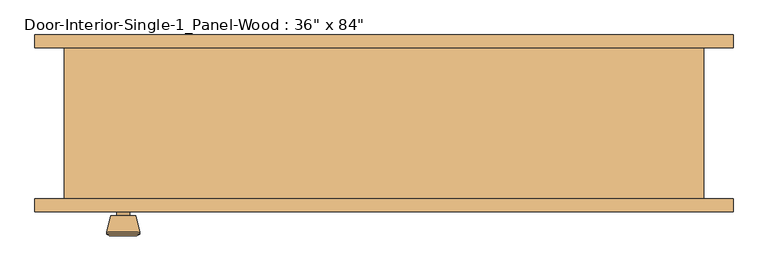
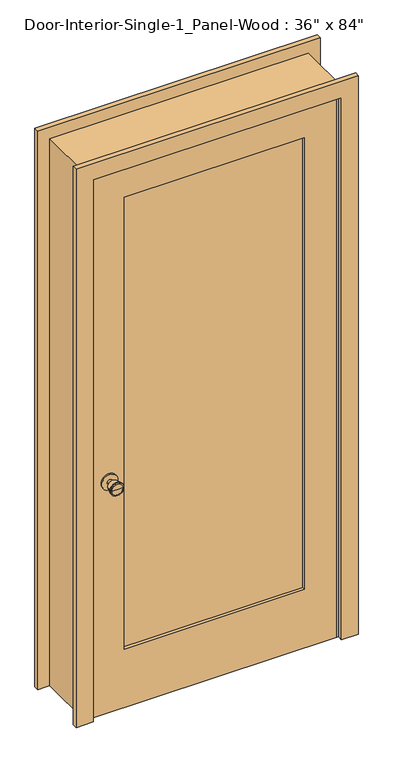
"""IFC4 building model written with IfcOpenShell, lengths in millimetres: door geometry."""

from ifc_helpers import new_model, si_unit, point, frame, frame_2d, origin, place, context, project, spatial, polyline, circle_curve, trimmed, segment, composite_curve, outline, extrude, faceted_brep, source, transform, mapped, element, save
from ifc_brep_helpers import plane_surface, cylinder_surface, revolved_surface, advanced_brep


def door_868ee8a9(model_context):
    return source(origin(), model_context, "Body", "SolidModel", [
        advanced_brep(
        [(-393.7, -70.2, 914.4), (-403.7, -70.2, 914.4), (-383.7, -70.2, 914.4), (-373.2241324, -21.2, 914.4), (-414.1758676, -21.2, 914.4), (-393.7, -21.2, 914.4), (-368.7, -23.0278681, 914.4), (-418.7, -23.0278681, 914.4), (-368.7, -26.4915463, 914.4), (-418.7, -26.4915463, 914.4), (-375.063764, -51.2, 914.4), (-412.336236, -51.2, 914.4), (-383.7, -51.2, 914.4), (-403.7, -51.2, 914.4)],
        [
            (0, 1),
            (1, 2, circle_curve(frame((-393.7, -70.2, 914.4), z_axis=(0.0, -1.0, 0.0), x_axis=(-1.0, 0.0, 0.0)), 10.0)),
            (2, 0),
            (2, 1, circle_curve(frame((-393.7, -70.2, 914.4), z_axis=(0.0, -1.0, 0.0), x_axis=(-1.0, 0.0, 0.0)), 10.0)),
            (3, 4, circle_curve(frame((-393.7, -21.2, 914.4), z_axis=(0.0, 1.0, 0.0), x_axis=(-1.0, 0.0, 0.0)), 20.4758676)),
            (4, 5),
            (5, 3),
            (4, 3, circle_curve(frame((-393.7, -21.2, 914.4), z_axis=(0.0, 1.0, 0.0), x_axis=(-1.0, 0.0, 0.0)), 20.4758676)),
            (6, 7, circle_curve(frame((-393.7, -23.0278681, 914.4), z_axis=(0.0, 1.0, 0.0), x_axis=(-1.0, 0.0, 0.0)), 25.0)),
            (7, 4),
            (3, 6),
            (7, 6, circle_curve(frame((-393.7, -23.0278681, 914.4), z_axis=(0.0, 1.0, 0.0), x_axis=(-1.0, 0.0, 0.0)), 25.0)),
            (8, 9, circle_curve(frame((-393.7, -26.4915463, 914.4), z_axis=(0.0, 1.0, 0.0), x_axis=(-1.0, 0.0, 0.0)), 25.0)),
            (9, 7),
            (6, 8),
            (9, 8, circle_curve(frame((-393.7, -26.4915463, 914.4), z_axis=(0.0, 1.0, 0.0), x_axis=(-1.0, 0.0, 0.0)), 25.0)),
            (10, 11, circle_curve(frame((-393.7, -51.2, 914.4), z_axis=(0.0, 1.0, 0.0), x_axis=(-1.0, 0.0, 0.0)), 18.636236)),
            (11, 9),
            (8, 10),
            (11, 10, circle_curve(frame((-393.7, -51.2, 914.4), z_axis=(0.0, 1.0, 0.0), x_axis=(-1.0, 0.0, 0.0)), 18.636236)),
            (12, 13, circle_curve(frame((-393.7, -51.2, 914.4), z_axis=(0.0, 1.0, 0.0), x_axis=(-1.0, 0.0, 0.0)), 10.0)),
            (13, 11),
            (10, 12),
            (13, 12, circle_curve(frame((-393.7, -51.2, 914.4), z_axis=(0.0, 1.0, 0.0), x_axis=(-1.0, 0.0, 0.0)), 10.0)),
            (1, 13),
            (12, 2),
        ],
        [
            plane_surface(frame((-393.7, -70.2, 914.4), z_axis=(0.0, -1.0, 0.0), x_axis=(-1.0, 0.0, 0.0))),
            plane_surface(frame((-393.7, -21.2, 914.4), z_axis=(0.0, 1.0, 0.0), x_axis=(-1.0, 0.0, 0.0))),
            revolved_surface(polyline([(-414.1758676, -21.2, 914.4), (-418.7, -23.0278681, 914.4)]), (-393.7, -70.2, 914.4), (0.0, -1.0, 0.0)),
            cylinder_surface(frame((-393.7, -70.2, 914.4), z_axis=(0.0, -1.0, 0.0), x_axis=(-1.0, 0.0, 0.0)), 25.0),
            revolved_surface(polyline([(-418.7, -26.4915463, 914.4), (-412.336236, -51.2, 914.4)]), (-393.7, -70.2, 914.4), (0.0, -1.0, 0.0)),
            plane_surface(frame((-393.7, -51.2, 914.4), z_axis=(0.0, -1.0, 0.0), x_axis=(-1.0, 0.0, 0.0))),
            cylinder_surface(frame((-393.7, -70.2, 914.4), z_axis=(0.0, -1.0, 0.0), x_axis=(-1.0, 0.0, 0.0)), 10.0),
        ],
        [
            (0, [[1, 2, 3]]),
            (0, [[-3, 4, -1]]),
            (1, [[5, 6, 7]]),
            (1, [[8, -7, -6]]),
            (2, [[9, 10, -5, 11]]),
            (2, [[12, -11, -8, -10]]),
            (3, [[13, 14, -9, 15]]),
            (3, [[16, -15, -12, -14]]),
            (4, [[17, 18, -13, 19]]),
            (4, [[20, -19, -16, -18]]),
            (5, [[21, 22, -17, 23]]),
            (5, [[24, -23, -20, -22]]),
            (6, [[-2, 25, -21, 26]]),
            (6, [[-4, -26, -24, -25]]),
        ],
    ),
        extrude(outline(composite_curve([segment(trimmed(circle_curve(frame_2d((914.4, -393.7)), 30.0), [point((914.4, -423.7))], [point((914.4, -363.7))], False, "CARTESIAN"), True, "CONTINUOUS"), segment(trimmed(circle_curve(frame_2d((914.4, -393.7)), 30.0), [point((914.4, -363.7))], [point((914.4, -423.7))], False, "CARTESIAN"), True, "CONTINUOUS")], self_intersect=False)), frame((0.0, -76.2, 0.0), z_axis=(0.0, 1.0, 0.0), x_axis=(0.0, 0.0, 1.0)), (0.0, 0.0, 1.0), 6.0),
        advanced_brep(
        [(-393.7, -117.125, 914.4), (-383.7, -117.125, 914.4), (-403.7, -117.125, 914.4), (-373.2241324, -166.125, 914.4), (-393.7, -166.125, 914.4), (-414.1758676, -166.125, 914.4), (-368.7, -164.2971319, 914.4), (-418.7, -164.2971319, 914.4), (-368.7, -160.8334537, 914.4), (-418.7, -160.8334537, 914.4), (-375.063764, -136.125, 914.4), (-412.336236, -136.125, 914.4), (-383.7, -136.125, 914.4), (-403.7, -136.125, 914.4)],
        [
            (0, 1),
            (1, 2, circle_curve(frame((-393.7, -117.125, 914.4), z_axis=(0.0, 1.0, 0.0), x_axis=(-1.0, 0.0, 0.0)), 10.0)),
            (2, 0),
            (2, 1, circle_curve(frame((-393.7, -117.125, 914.4), z_axis=(0.0, 1.0, 0.0), x_axis=(-1.0, 0.0, 0.0)), 10.0)),
            (3, 4),
            (4, 5),
            (5, 3, circle_curve(frame((-393.7, -166.125, 914.4), z_axis=(0.0, -1.0, 0.0), x_axis=(-1.0, 0.0, 0.0)), 20.4758676)),
            (3, 5, circle_curve(frame((-393.7, -166.125, 914.4), z_axis=(0.0, -1.0, 0.0), x_axis=(-1.0, 0.0, 0.0)), 20.4758676)),
            (6, 3),
            (5, 7),
            (7, 6, circle_curve(frame((-393.7, -164.2971319, 914.4), z_axis=(0.0, -1.0, 0.0), x_axis=(-1.0, 0.0, 0.0)), 25.0)),
            (6, 7, circle_curve(frame((-393.7, -164.2971319, 914.4), z_axis=(0.0, -1.0, 0.0), x_axis=(-1.0, 0.0, 0.0)), 25.0)),
            (8, 6),
            (7, 9),
            (9, 8, circle_curve(frame((-393.7, -160.8334537, 914.4), z_axis=(0.0, -1.0, 0.0), x_axis=(-1.0, 0.0, 0.0)), 25.0)),
            (8, 9, circle_curve(frame((-393.7, -160.8334537, 914.4), z_axis=(0.0, -1.0, 0.0), x_axis=(-1.0, 0.0, 0.0)), 25.0)),
            (10, 8),
            (9, 11),
            (11, 10, circle_curve(frame((-393.7, -136.125, 914.4), z_axis=(0.0, -1.0, 0.0), x_axis=(-1.0, 0.0, 0.0)), 18.636236)),
            (10, 11, circle_curve(frame((-393.7, -136.125, 914.4), z_axis=(0.0, -1.0, 0.0), x_axis=(-1.0, 0.0, 0.0)), 18.636236)),
            (12, 10),
            (11, 13),
            (13, 12, circle_curve(frame((-393.7, -136.125, 914.4), z_axis=(0.0, -1.0, 0.0), x_axis=(-1.0, 0.0, 0.0)), 10.0)),
            (12, 13, circle_curve(frame((-393.7, -136.125, 914.4), z_axis=(0.0, -1.0, 0.0), x_axis=(-1.0, 0.0, 0.0)), 10.0)),
            (1, 12),
            (13, 2),
        ],
        [
            plane_surface(frame((-393.7, -117.125, 914.4), z_axis=(0.0, 1.0, 0.0), x_axis=(-1.0, 0.0, 0.0))),
            plane_surface(frame((-393.7, -166.125, 914.4), z_axis=(0.0, -1.0, 0.0), x_axis=(-1.0, 0.0, 0.0))),
            revolved_surface(polyline([(-414.1758676, -166.125, 914.4), (-418.7, -164.2971319, 914.4)]), (-393.7, -117.125, 914.4), (0.0, 1.0, 0.0)),
            cylinder_surface(frame((-393.7, -117.125, 914.4), z_axis=(0.0, 1.0, 0.0), x_axis=(-1.0, 0.0, 0.0)), 25.0),
            revolved_surface(polyline([(-418.7, -160.8334537, 914.4), (-412.336236, -136.125, 914.4)]), (-393.7, -117.125, 914.4), (0.0, 1.0, 0.0)),
            plane_surface(frame((-393.7, -136.125, 914.4), z_axis=(0.0, 1.0, 0.0), x_axis=(-1.0, 0.0, 0.0))),
            cylinder_surface(frame((-393.7, -117.125, 914.4), z_axis=(0.0, 1.0, 0.0), x_axis=(-1.0, 0.0, 0.0)), 10.0),
        ],
        [
            (0, [[1, 2, 3]]),
            (0, [[-3, 4, -1]]),
            (1, [[5, 6, 7]]),
            (1, [[-6, -5, 8]]),
            (2, [[9, -7, 10, 11]]),
            (2, [[-10, -8, -9, 12]]),
            (3, [[13, -11, 14, 15]]),
            (3, [[-14, -12, -13, 16]]),
            (4, [[17, -15, 18, 19]]),
            (4, [[-18, -16, -17, 20]]),
            (5, [[21, -19, 22, 23]]),
            (5, [[-22, -20, -21, 24]]),
            (6, [[25, -23, 26, -2]]),
            (6, [[-26, -24, -25, -4]]),
        ],
    ),
        extrude(outline(composite_curve([segment(trimmed(circle_curve(frame_2d((914.4, -393.7)), 30.0), [point((914.4, -423.7))], [point((914.4, -363.7))], False, "CARTESIAN"), True, "CONTINUOUS"), segment(trimmed(circle_curve(frame_2d((914.4, -393.7)), 30.0), [point((914.4, -363.7))], [point((914.4, -423.7))], False, "CARTESIAN"), True, "CONTINUOUS")], self_intersect=False)), frame((0.0, -117.125, 0.0), z_axis=(0.0, 1.0, 0.0), x_axis=(0.0, 0.0, 1.0)), (0.0, 0.0, 1.0), 6.0),
        faceted_brep([(482.6, -111.125, 0.0), (457.2, -111.125, 0.0), (457.2, -76.2, 0.0), (444.5, -76.2, 0.0), (444.5, -41.275, 0.0), (457.2, -41.275, 0.0), (457.2, 117.475, 0.0), (482.6, 117.475, 0.0), (482.6, 117.475, 2159.0), (482.6, -111.125, 2159.0), (457.2, 117.475, 2133.6), (-457.2, 117.475, 2133.6), (-457.2, 117.475, 0.0), (-482.6, 117.475, 0.0), (-482.6, 117.475, 2159.0), (457.2, -41.275, 2133.6), (444.5, -41.275, 2120.9), (-444.5, -41.275, 2120.9), (-444.5, -41.275, 0.0), (-457.2, -41.275, 0.0), (-457.2, -41.275, 2133.6), (444.5, -76.2, 2120.9), (457.2, -76.2, 2133.6), (-457.2, -76.2, 2133.6), (-457.2, -76.2, 0.0), (-444.5, -76.2, 0.0), (-444.5, -76.2, 2120.9), (457.2, -111.125, 2133.6), (-482.6, -111.125, 2159.0), (-482.6, -111.125, 0.0), (-457.2, -111.125, 0.0), (-457.2, -111.125, 2133.6)], [[[0, 1, 2, 3, 4, 5, 6, 7]], [[7, 8, 9, 0]], [[6, 10, 11, 12, 13, 14, 8, 7]], [[5, 15, 10, 6]], [[4, 16, 17, 18, 19, 20, 15, 5]], [[3, 21, 16, 4]], [[2, 22, 23, 24, 25, 26, 21, 3]], [[1, 27, 22, 2]], [[0, 9, 28, 29, 30, 31, 27, 1]], [[8, 14, 28, 9]], [[15, 20, 11, 10]], [[21, 26, 17, 16]], [[27, 31, 23, 22]], [[29, 13, 12, 19, 18, 25, 24, 30]], [[14, 13, 29, 28]], [[20, 19, 12, 11]], [[26, 25, 18, 17]], [[31, 30, 24, 23]]]),
        extrude(outline(polyline([(2133.6, -457.2), (0.0, -457.2), (0.0, 457.2), (2133.6, 457.2), (2133.6, -457.2)]), holes=[polyline([(2014.5375, -336.55), (2014.5375, 336.55), (231.775, 336.55), (231.775, -336.55), (2014.5375, -336.55)])]), frame((0.0, -111.125, 0.0), z_axis=(0.0, 1.0, 0.0), x_axis=(0.0, 0.0, 1.0)), (0.0, 0.0, 1.0), 34.925),
        extrude(outline(polyline([(336.55, -87.8416667), (336.55, -99.4833333), (-336.55, -99.4833333), (-336.55, -87.8416667), (336.55, -87.8416667)])), frame((0.0, 0.0, 231.775), z_axis=(0.0, 0.0, 1.0), x_axis=(1.0, 0.0, 0.0)), (0.0, 0.0, 1.0), 1782.7625),
        extrude(outline(polyline([(0.0, 527.05), (2203.45, 527.05), (2203.45, -527.05), (0.0, -527.05), (0.0, -463.55), (2139.95, -463.55), (2139.95, 463.55), (0.0, 463.55), (0.0, 527.05)])), frame((0.0, -130.175, 0.0), z_axis=(0.0, 1.0, 0.0), x_axis=(0.0, 0.0, 1.0)), (0.0, 0.0, 1.0), 19.05),
        extrude(outline(polyline([(0.0, 527.05), (2203.45, 527.05), (2203.45, -527.05), (0.0, -527.05), (0.0, -463.55), (2139.95, -463.55), (2139.95, 463.55), (0.0, 463.55), (0.0, 527.05)])), frame((0.0, 117.475, 0.0), z_axis=(0.0, 1.0, 0.0), x_axis=(0.0, 0.0, 1.0)), (0.0, 0.0, 1.0), 19.05),
    ])


if __name__ == "__main__":
    model = new_model("IFC4")
    model_context = context("Model", 3, world=origin())
    ifc_project = project(units=[si_unit("LENGTHUNIT", "METRE", prefix="MILLI")], contexts=[model_context])
    site = spatial("IfcSite", under=ifc_project)
    building = spatial("IfcBuilding", under=site)
    placement = place(None, origin())
    door_shape = door_868ee8a9(model_context)
    element("IfcDoor", 1, ObjectType="Door-Interior-Single-1_Panel-Wood : 36\" x 84\"", at=placement, inside=building, context=model_context, shape_type="MappedRepresentation", body=[
        mapped(door_shape, transform((0.0, 0.0, 0.0), x_axis=(1.0, 0.0, 0.0), y_axis=(0.0, 1.0, 0.0), z_axis=(0.0, 0.0, 1.0))),
    ])
    save(model, "model.ifc")

# Revit data of these elements
# Type "Door-Interior-Single-1_Panel-Wood : 36\" x 84\""
#   Type Mark = "8"
#   Assembly Code = "C1020300"
#   Analytic Construction = "Wooden"
#   Top Rail = 0' - 4 11/16"
#   Thickness = 0' - 1 3/8"
#   Thermal Resistance (R) = 2.5876 (h·ft²·°F)/BTU
#   Swing Angle [instance default] = 90.00°
#   Stiles = 0' - 4 3/4"
#   Rough Width = 3' - 2"
#   Rough Height = 7' - 1"
#   Height = 7' - 0"
#   Width = 3' - 0"
#   Heat Transfer Coefficient (U) = 0.3865 BTU/(h·ft²·°F)
#   Bottom Rail = 0' - 9 1/8"
#   Trim Material = Cherry
#   Panel Material = Cherry
#   Frame Material = Cherry
#   Door Handle Material = Aluminum
#   Visual Light Transmittance = 0
#   Solar Heat Gain Coefficient = 0
#   Wall Closure = (empty or 0)
#   Function = (empty or 0)
# Element 1 (IfcDoor, "Door-Interior-Single-1_Panel-Wood : 36\" x 84\"")
#   Materials on its faces: "Cherry", "Aluminum"
# Materials
#   "Cherry": class "Wood", colour RGB 226 177 128, transparency 0, Description = "Prunus Serotina", Cost = 0
#   "Aluminum": class "Metal", colour RGB 247 247 247, transparency 0, Description = "Aluminum 6061", Cost = 0
